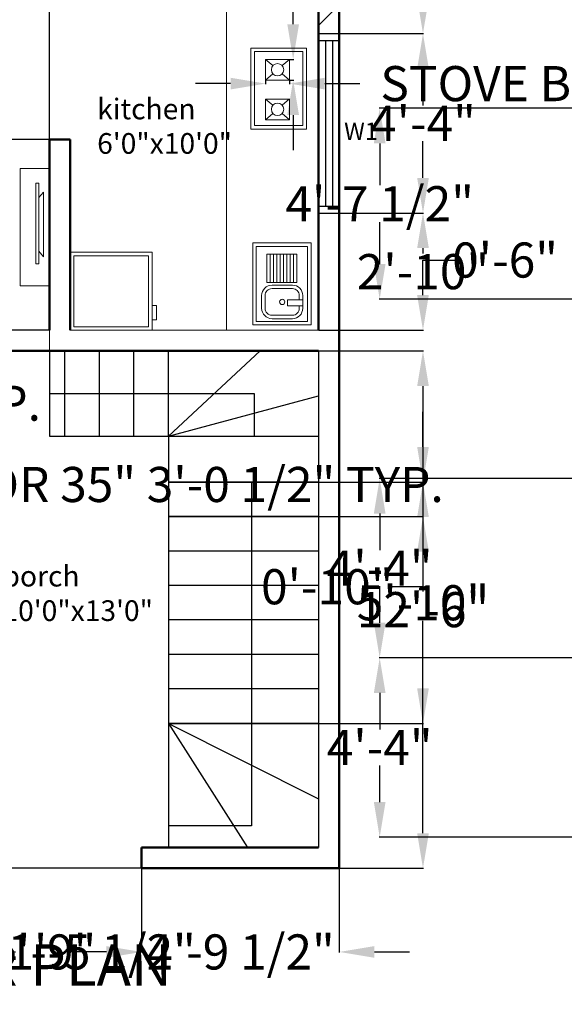
# Model space of a CAD drawing. Units: inches. Extents: x 21 to 3450, y 4 to 2137.
# Tile 10 of 14: x 2964 to 3122, y 1047 to 1333. Entities that reach past the tile are written whole.
import ezdxf

# ---------------------------------------------------------------- set-up
doc = ezdxf.new("R2010")
doc.units = ezdxf.units.IN
doc.header["$MEASUREMENT"] = 0
for name, color, linetype, lineweight in [('A-ANNO-DIMS', 2, 'Continuous', 18), ('A-ANNO-TEXT', 7, 'Continuous', 18), ('A-AREA-IDEN', 3, 'Continuous', 18), ('A-FLOR-FIXT', 9, 'Continuous', 18), ('A-FLOR-STRS', 2, 'Continuous', 25), ('A-FURN', 8, 'Continuous', 18), ('A-GLAZ', 3, 'Continuous', 25), ('A-WALL', 7, 'Continuous', 50), ('A-WALL-PATT', 8, 'Continuous', 13)]:
    doc.layers.add(name, color=color, linetype=linetype, lineweight=lineweight)
doc.styles.get("Standard").update_dxf_attribs({"font": 'arial.ttf'})
doc.dimstyles.get("Standard").update_dxf_attribs({"dimtxt": 10.18, "dimasz": 10.18, "dimexe": 0.18, "dimexo": 0.0625, "dimgap": 0.09, "dimtad": 0, "dimtih": 1, "dimtoh": 1, "dimdec": 0, "dimzin": 0, "dimdsep": 46, "dimlunit": 3, "dimtxsty": 'Standard', "dimcen": 0.09, "dimadec": 0, "dimazin": 0, "dimtfac": 1, "dimtdec": 0, "dimtofl": 0, "dimtmove": 0, "dimatfit": 3, "dimfxl": 1, "dimtolj": 1, "dimtzin": 0, "dimarcsym": 0})

# ---------------------------------------------------------------- blocks, each defined once
blk = doc.blocks.new('*D8')
at = {"layer": 'A-ANNO-DIMS', "color": 0, "lineweight": -2, "transparency": 16777216}
for p, q in [((2816.85, 1506.81), (2803.73, 1506.81)), ((2803.91, 1496.63), (2803.91, 1302.07)), ((2803.91, 1096.92), (2803.91, 1291.48)), ((2999.5, 1086.74), (2803.73, 1086.74))]:
    blk.add_line(p, q, dxfattribs=at)
at = {"layer": 'A-ANNO-DIMS', "color": 0, "transparency": 16777216}
for points in [[(2802.22, 1496.63), (2805.61, 1496.63), (2803.91, 1506.81)], [(2802.22, 1096.92), (2805.61, 1096.92), (2803.91, 1086.74)]]:
    blk.add_solid(points, dxfattribs=at)
at = {"layer": 'Defpoints', "color": 0, "transparency": 16777216}
for p in [(2816.91, 1506.81), (2803.91, 1086.74), (2999.56, 1086.74)]:
    blk.add_point(p, dxfattribs=at)
at = {"layer": 'A-ANNO-DIMS', "color": 0, "transparency": 16777216, "insert": (2803.91, 1296.77), "char_height": 10.18, "attachment_point": 5}
blk.add_mtext("\\A1;35'", dxfattribs=at)
blk = doc.blocks.new('STOVE-BURNER')
blk.add_line((0, 5.99), (2.12, 4.17))
blk.add_lwpolyline([(0, 5.99), (0, 5.99), (6.94, 5.99), (6.94, 5.99), (6.94, 0), (6.94, 0), (0, 0), (0, 0)], close=True)
blk = doc.blocks.new('*D26')
at = {"layer": 'A-ANNO-DIMS', "color": 0, "lineweight": -2, "transparency": 16777216}
for p, q in [((2885.64, 1203.41), (2885.64, 1197.85)), ((2921.91, 1203.41), (2921.91, 1197.85)), ((2895.82, 1198.03), (2911.73, 1198.03)), ((2921.91, 1198.03), (2932.09, 1198.03))]:
    blk.add_line(p, q, dxfattribs=at)
at = {"layer": 'A-ANNO-DIMS', "color": 0, "transparency": 16777216}
for points in [[(2895.82, 1199.72), (2895.82, 1196.33), (2885.64, 1198.03)], [(2911.73, 1199.72), (2911.73, 1196.33), (2921.91, 1198.03)]]:
    blk.add_solid(points, dxfattribs=at)
at = {"layer": 'Defpoints', "color": 0, "transparency": 16777216}
for p in [(2885.64, 1203.47), (2921.91, 1203.47), (2921.91, 1198.03)]:
    blk.add_point(p, dxfattribs=at)
at = {"layer": 'A-ANNO-DIMS', "color": 0, "transparency": 16777216, "insert": (3010.53, 1198.03), "char_height": 10.18, "attachment_point": 5}
blk.add_mtext('\\A1;DOOR 35" 3\'-0 1/2" TYP.', dxfattribs=at)
blk = doc.blocks.new('*D27')
at = {"layer": 'A-ANNO-DIMS', "color": 0, "lineweight": -2, "transparency": 16777216}
for p, q in [((2921.97, 1239.74), (2927.53, 1239.74)), ((2927.35, 1229.56), (2927.35, 1226.96)), ((2927.35, 1213.65), (2927.35, 1216.25)), ((2921.97, 1203.47), (2927.53, 1203.47))]:
    blk.add_line(p, q, dxfattribs=at)
at = {"layer": 'A-ANNO-DIMS', "color": 0, "transparency": 16777216}
for points in [[(2925.66, 1229.56), (2929.05, 1229.56), (2927.35, 1239.74)], [(2925.66, 1213.65), (2929.05, 1213.65), (2927.35, 1203.47)]]:
    blk.add_solid(points, dxfattribs=at)
at = {"layer": 'Defpoints', "color": 0, "transparency": 16777216}
for p in [(2921.91, 1239.74), (2927.35, 1239.74), (2921.91, 1203.47)]:
    blk.add_point(p, dxfattribs=at)
at = {"layer": 'A-ANNO-DIMS', "color": 0, "transparency": 16777216, "insert": (2927.35, 1221.61), "char_height": 10.18, "attachment_point": 5}
blk.add_mtext('\\A1;3\'-0 1/2" TYP.', dxfattribs=at)
blk = doc.blocks.new('*D32')
at = {"layer": 'A-ANNO-DIMS', "color": 0, "lineweight": -2, "transparency": 16777216}
for p, q in [((3025.36, 1314.25), (3015.18, 1314.25)), ((3035.54, 1315.23), (3035.54, 1314.07)), ((3042.48, 1315.23), (3042.48, 1314.07)), ((3052.66, 1314.25), (3062.84, 1314.25))]:
    blk.add_line(p, q, dxfattribs=at)
at = {"layer": 'A-ANNO-DIMS', "color": 0, "transparency": 16777216}
for points in [[(3025.36, 1315.95), (3025.36, 1312.56), (3035.54, 1314.25)], [(3052.66, 1315.95), (3052.66, 1312.56), (3042.48, 1314.25)]]:
    blk.add_solid(points, dxfattribs=at)
at = {"layer": 'Defpoints', "color": 0, "transparency": 16777216}
for p in [(3035.54, 1315.29), (3042.48, 1315.29), (3042.48, 1314.25)]:
    blk.add_point(p, dxfattribs=at)
at = {"layer": 'A-ANNO-DIMS', "color": 0, "transparency": 16777216, "insert": (3152.02, 1314.25), "char_height": 10.18, "attachment_point": 5}
blk.add_mtext('\\A1;STOVE BURNER 0\'-7" TYP.', dxfattribs=at)
blk = doc.blocks.new('*D33')
at = {"layer": 'A-ANNO-DIMS', "color": 0, "lineweight": -2, "transparency": 16777216}
for p, q in [((3043.53, 1331.47), (3043.53, 1341.65)), ((3043.53, 1341.65), (3053.71, 1341.65)), ((3042.55, 1321.29), (3043.71, 1321.29)), ((3042.55, 1315.29), (3043.71, 1315.29)), ((3043.53, 1305.11), (3043.53, 1294.93))]:
    blk.add_line(p, q, dxfattribs=at)
at = {"layer": 'A-ANNO-DIMS', "color": 0, "transparency": 16777216}
for points in [[(3041.83, 1331.47), (3045.22, 1331.47), (3043.53, 1321.29)], [(3041.83, 1305.11), (3045.22, 1305.11), (3043.53, 1315.29)]]:
    blk.add_solid(points, dxfattribs=at)
at = {"layer": 'Defpoints', "color": 0, "transparency": 16777216}
for p in [(3042.48, 1321.29), (3043.53, 1321.29), (3042.48, 1315.29)]:
    blk.add_point(p, dxfattribs=at)
at = {"layer": 'A-ANNO-DIMS', "color": 0, "transparency": 16777216, "insert": (3084.82, 1341.65), "char_height": 10.18, "attachment_point": 5}
blk.add_mtext('\\A1;0\'-6" TYP.', dxfattribs=at)
blk = doc.blocks.new('*D104')
at = {"layer": 'A-ANNO-DIMS', "color": 0, "lineweight": -2, "transparency": 16777216}
for p, q in [((2924.91, 1092.68), (2924.91, 1062.31)), ((2942.64, 1086.68), (2942.64, 1062.31)), ((2914.73, 1062.49), (2904.55, 1062.49)), ((2952.82, 1062.49), (2963, 1062.49))]:
    blk.add_line(p, q, dxfattribs=at)
at = {"layer": 'A-ANNO-DIMS', "color": 0, "transparency": 16777216}
for points in [[(2914.73, 1064.19), (2914.73, 1060.8), (2924.91, 1062.49)], [(2952.82, 1064.19), (2952.82, 1060.8), (2942.64, 1062.49)]]:
    blk.add_solid(points, dxfattribs=at)
at = {"layer": 'Defpoints', "color": 0, "transparency": 16777216}
for p in [(2924.91, 1092.74), (2942.64, 1086.74), (2942.64, 1062.49)]:
    blk.add_point(p, dxfattribs=at)
at = {"layer": 'A-ANNO-DIMS', "color": 0, "transparency": 16777216, "insert": (2988, 1062.49), "char_height": 10.18, "attachment_point": 5}
blk.add_mtext('\\A1;1\'-5 1/2"', dxfattribs=at)
blk = doc.blocks.new('*D105')
at = {"layer": 'A-ANNO-DIMS', "color": 0, "lineweight": -2, "transparency": 16777216}
for p, q in [((2942.64, 1086.68), (2942.64, 1062.31)), ((2999.56, 1086.68), (2999.56, 1062.31)), ((2952.82, 1062.49), (2957.27, 1062.49)), ((2989.38, 1062.49), (2984.92, 1062.49))]:
    blk.add_line(p, q, dxfattribs=at)
at = {"layer": 'A-ANNO-DIMS', "color": 0, "transparency": 16777216}
for points in [[(2952.82, 1064.19), (2952.82, 1060.8), (2942.64, 1062.49)], [(2989.38, 1064.19), (2989.38, 1060.8), (2999.56, 1062.49)]]:
    blk.add_solid(points, dxfattribs=at)
at = {"layer": 'Defpoints', "color": 0, "transparency": 16777216}
for p in [(2942.64, 1086.74), (2999.56, 1086.74), (2999.56, 1062.49)]:
    blk.add_point(p, dxfattribs=at)
at = {"layer": 'A-ANNO-DIMS', "color": 0, "transparency": 16777216, "insert": (2971.1, 1062.49), "char_height": 10.18, "attachment_point": 5}
blk.add_mtext('\\A1;4\'-9"', dxfattribs=at)
blk = doc.blocks.new('*D106')
at = {"layer": 'A-ANNO-DIMS', "color": 0, "lineweight": -2, "transparency": 16777216}
for p, q in [((2999.56, 1086.68), (2999.56, 1062.31)), ((3056.91, 1086.68), (3056.91, 1062.31)), ((2989.38, 1062.49), (2979.2, 1062.49)), ((3067.09, 1062.49), (3077.27, 1062.49))]:
    blk.add_line(p, q, dxfattribs=at)
at = {"layer": 'A-ANNO-DIMS', "color": 0, "transparency": 16777216}
for points in [[(2989.38, 1064.19), (2989.38, 1060.8), (2999.56, 1062.49)], [(3067.09, 1064.19), (3067.09, 1060.8), (3056.91, 1062.49)]]:
    blk.add_solid(points, dxfattribs=at)
at = {"layer": 'Defpoints', "color": 0, "transparency": 16777216}
for p in [(2999.56, 1086.74), (3056.91, 1086.74), (3056.91, 1062.49)]:
    blk.add_point(p, dxfattribs=at)
at = {"layer": 'A-ANNO-DIMS', "color": 0, "transparency": 16777216, "insert": (3028.24, 1062.49), "char_height": 10.18, "attachment_point": 5}
blk.add_mtext('\\A1;4\'-9 1/2"', dxfattribs=at)
blk = doc.blocks.new('*D107')
at = {"layer": 'A-ANNO-DIMS', "color": 0, "lineweight": -2, "transparency": 16777216}
for p, q in [((3050.97, 1236.74), (3081.34, 1236.74)), ((3081.16, 1226.56), (3081.16, 1167.03)), ((3081.16, 1096.92), (3081.16, 1156.46)), ((3056.97, 1086.74), (3081.34, 1086.74))]:
    blk.add_line(p, q, dxfattribs=at)
at = {"layer": 'A-ANNO-DIMS', "color": 0, "transparency": 16777216}
for points in [[(3079.47, 1226.56), (3082.86, 1226.56), (3081.16, 1236.74)], [(3079.47, 1096.92), (3082.86, 1096.92), (3081.16, 1086.74)]]:
    blk.add_solid(points, dxfattribs=at)
at = {"layer": 'Defpoints', "color": 0, "transparency": 16777216}
for p in [(3050.91, 1236.74), (3081.16, 1236.74), (3056.91, 1086.74)]:
    blk.add_point(p, dxfattribs=at)
at = {"layer": 'A-ANNO-DIMS', "color": 0, "transparency": 16777216, "insert": (3081.16, 1161.74), "char_height": 10.18, "attachment_point": 5}
blk.add_mtext('\\A1;12\'-6"', dxfattribs=at)
blk = doc.blocks.new('*D108')
at = {"layer": 'A-ANNO-DIMS', "color": 0, "lineweight": -2, "transparency": 16777216}
for p, q in [((3081.16, 1252.92), (3081.16, 1263.1)), ((3081.16, 1263.1), (3091.34, 1263.1)), ((3050.97, 1242.74), (3081.34, 1242.74)), ((3050.97, 1236.74), (3081.34, 1236.74)), ((3081.16, 1226.56), (3081.16, 1216.38))]:
    blk.add_line(p, q, dxfattribs=at)
at = {"layer": 'A-ANNO-DIMS', "color": 0, "transparency": 16777216}
for points in [[(3079.47, 1252.92), (3082.86, 1252.92), (3081.16, 1242.74)], [(3079.47, 1226.56), (3082.86, 1226.56), (3081.16, 1236.74)]]:
    blk.add_solid(points, dxfattribs=at)
at = {"layer": 'Defpoints', "color": 0, "transparency": 16777216}
for p in [(3050.91, 1242.74), (3081.16, 1242.74), (3050.91, 1236.74)]:
    blk.add_point(p, dxfattribs=at)
at = {"layer": 'A-ANNO-DIMS', "color": 0, "transparency": 16777216, "insert": (3104.96, 1263.1), "char_height": 10.18, "attachment_point": 5}
blk.add_mtext('\\A1;0\'-6"', dxfattribs=at)
blk = doc.blocks.new('*D109')
at = {"layer": 'A-ANNO-DIMS', "color": 0, "lineweight": -2, "transparency": 16777216}
for p, q in [((3056.97, 1276.74), (3081.34, 1276.74)), ((3081.16, 1266.56), (3081.16, 1265.03)), ((3081.16, 1252.92), (3081.16, 1254.46)), ((3050.97, 1242.74), (3081.34, 1242.74))]:
    blk.add_line(p, q, dxfattribs=at)
at = {"layer": 'A-ANNO-DIMS', "color": 0, "transparency": 16777216}
for points in [[(3079.47, 1266.56), (3082.86, 1266.56), (3081.16, 1276.74)], [(3079.47, 1252.92), (3082.86, 1252.92), (3081.16, 1242.74)]]:
    blk.add_solid(points, dxfattribs=at)
at = {"layer": 'Defpoints', "color": 0, "transparency": 16777216}
for p in [(3056.91, 1276.74), (3081.16, 1276.74), (3050.91, 1242.74)]:
    blk.add_point(p, dxfattribs=at)
at = {"layer": 'A-ANNO-DIMS', "color": 0, "transparency": 16777216, "insert": (3081.16, 1259.74), "char_height": 10.18, "attachment_point": 5}
blk.add_mtext('\\A1;2\'-10"', dxfattribs=at)
blk = doc.blocks.new('*D110')
at = {"layer": 'A-ANNO-DIMS', "color": 0, "lineweight": -2, "transparency": 16777216}
for p, q in [((3056.97, 1328.74), (3081.34, 1328.74)), ((3081.16, 1318.56), (3081.16, 1307.92)), ((3081.16, 1286.92), (3081.16, 1297.56)), ((3056.97, 1276.74), (3081.34, 1276.74))]:
    blk.add_line(p, q, dxfattribs=at)
at = {"layer": 'A-ANNO-DIMS', "color": 0, "transparency": 16777216}
for points in [[(3079.47, 1318.56), (3082.86, 1318.56), (3081.16, 1328.74)], [(3079.47, 1286.92), (3082.86, 1286.92), (3081.16, 1276.74)]]:
    blk.add_solid(points, dxfattribs=at)
at = {"layer": 'Defpoints', "color": 0, "transparency": 16777216}
for p in [(3056.91, 1328.74), (3081.16, 1328.74), (3056.91, 1276.74)]:
    blk.add_point(p, dxfattribs=at)
at = {"layer": 'A-ANNO-DIMS', "color": 0, "transparency": 16777216, "insert": (3081.16, 1302.74), "char_height": 10.18, "attachment_point": 5}
blk.add_mtext('\\A1;4\'-4"', dxfattribs=at)
blk = doc.blocks.new('*D111')
at = {"layer": 'A-ANNO-DIMS', "color": 0, "lineweight": -2, "transparency": 16777216}
for p, q in [((3050.97, 1362.74), (3081.34, 1362.74)), ((3081.16, 1352.56), (3081.16, 1351.03)), ((3081.16, 1338.92), (3081.16, 1340.46)), ((3056.97, 1328.74), (3081.34, 1328.74))]:
    blk.add_line(p, q, dxfattribs=at)
at = {"layer": 'A-ANNO-DIMS', "color": 0, "transparency": 16777216}
for points in [[(3079.47, 1352.56), (3082.86, 1352.56), (3081.16, 1362.74)], [(3079.47, 1338.92), (3082.86, 1338.92), (3081.16, 1328.74)]]:
    blk.add_solid(points, dxfattribs=at)
at = {"layer": 'Defpoints', "color": 0, "transparency": 16777216}
for p in [(3050.91, 1362.74), (3081.16, 1362.74), (3056.91, 1328.74)]:
    blk.add_point(p, dxfattribs=at)
at = {"layer": 'A-ANNO-DIMS', "color": 0, "transparency": 16777216, "insert": (3081.16, 1345.74), "char_height": 10.18, "attachment_point": 5}
blk.add_mtext('\\A1;2\'-10"', dxfattribs=at)
blk = doc.blocks.new('*D118')
at = {"layer": 'A-ANNO-DIMS', "color": 0, "lineweight": -2, "transparency": 16777216}
for p, q in [((2920.73, 1539.16), (2910.55, 1539.16)), ((2930.91, 1242.81), (2930.91, 1539.34)), ((2972.91, 1242.81), (2972.91, 1539.34)), ((2983.09, 1539.16), (2993.27, 1539.16))]:
    blk.add_line(p, q, dxfattribs=at)
at = {"layer": 'A-ANNO-DIMS', "color": 0, "transparency": 16777216}
for points in [[(2920.73, 1540.85), (2920.73, 1537.46), (2930.91, 1539.16)], [(2983.09, 1540.85), (2983.09, 1537.46), (2972.91, 1539.16)]]:
    blk.add_solid(points, dxfattribs=at)
at = {"layer": 'Defpoints', "color": 0, "transparency": 16777216}
for p in [(2972.91, 1539.16), (2930.91, 1242.74), (2972.91, 1242.74)]:
    blk.add_point(p, dxfattribs=at)
at = {"layer": 'A-ANNO-DIMS', "color": 0, "transparency": 16777216, "insert": (2951.91, 1539.16), "char_height": 10.18, "attachment_point": 5}
blk.add_mtext('\\A1;3\'-6"', dxfattribs=at)
blk = doc.blocks.new('*D120')
at = {"layer": 'A-ANNO-DIMS', "color": 0, "lineweight": -2, "transparency": 16777216}
for p, q in [((2972.85, 1298.07), (2738.48, 1298.07)), ((2738.66, 1287.89), (2738.66, 1275.76)), ((2738.66, 1252.92), (2738.66, 1265.05)), ((2972.85, 1242.74), (2738.48, 1242.74))]:
    blk.add_line(p, q, dxfattribs=at)
at = {"layer": 'A-ANNO-DIMS', "color": 0, "transparency": 16777216}
for points in [[(2736.97, 1287.89), (2740.36, 1287.89), (2738.66, 1298.07)], [(2736.97, 1252.92), (2740.36, 1252.92), (2738.66, 1242.74)]]:
    blk.add_solid(points, dxfattribs=at)
at = {"layer": 'Defpoints', "color": 0, "transparency": 16777216}
for p in [(2738.66, 1298.07), (2972.91, 1298.07), (2972.91, 1242.74)]:
    blk.add_point(p, dxfattribs=at)
at = {"layer": 'A-ANNO-DIMS', "color": 0, "transparency": 16777216, "insert": (2738.66, 1270.41), "char_height": 10.18, "attachment_point": 5}
blk.add_mtext('\\A1;4\'-7 1/2"', dxfattribs=at)
blk = doc.blocks.new('*D121')
at = {"layer": 'A-ANNO-DIMS', "color": 0, "lineweight": -2, "transparency": 16777216}
for p, q in [((3081.16, 1208.92), (3081.16, 1219.1)), ((3007.42, 1198.74), (3081.34, 1198.74)), ((3007.42, 1188.74), (3081.34, 1188.74)), ((3081.16, 1178.56), (3081.16, 1168.38)), ((3081.16, 1168.38), (3070.98, 1168.38))]:
    blk.add_line(p, q, dxfattribs=at)
at = {"layer": 'A-ANNO-DIMS', "color": 0, "transparency": 16777216}
for points in [[(3079.47, 1208.92), (3082.86, 1208.92), (3081.16, 1198.74)], [(3079.47, 1178.56), (3082.86, 1178.56), (3081.16, 1188.74)]]:
    blk.add_solid(points, dxfattribs=at)
at = {"layer": 'Defpoints', "color": 0, "transparency": 16777216}
for p in [(3007.36, 1198.74), (3007.36, 1188.74), (3081.16, 1188.74)]:
    blk.add_point(p, dxfattribs=at)
at = {"layer": 'A-ANNO-DIMS', "color": 0, "transparency": 16777216, "insert": (3053.41, 1168.38), "char_height": 10.18, "attachment_point": 5}
blk.add_mtext('\\A1;0\'-10"', dxfattribs=at)
blk = doc.blocks.new('*D122')
at = {"layer": 'A-ANNO-DIMS', "color": 0, "lineweight": -2, "transparency": 16777216}
for p, q in [((3007.42, 1198.74), (3081.34, 1198.74)), ((3081.16, 1188.56), (3081.16, 1169.03)), ((3081.16, 1138.92), (3081.16, 1158.46)), ((3007.42, 1128.74), (3081.34, 1128.74))]:
    blk.add_line(p, q, dxfattribs=at)
at = {"layer": 'A-ANNO-DIMS', "color": 0, "transparency": 16777216}
for points in [[(3079.47, 1188.56), (3082.86, 1188.56), (3081.16, 1198.74)], [(3079.47, 1138.92), (3082.86, 1138.92), (3081.16, 1128.74)]]:
    blk.add_solid(points, dxfattribs=at)
at = {"layer": 'Defpoints', "color": 0, "transparency": 16777216}
for p in [(3007.36, 1198.74), (3007.36, 1128.74), (3081.16, 1128.74)]:
    blk.add_point(p, dxfattribs=at)
at = {"layer": 'A-ANNO-DIMS', "color": 0, "transparency": 16777216, "insert": (3081.16, 1163.74), "char_height": 10.18, "attachment_point": 5}
blk.add_mtext('\\A1;5\'-10"', dxfattribs=at)
blk = doc.blocks.new('*D141')
at = {"layer": 'A-ANNO-DIMS', "color": 0, "lineweight": -2, "transparency": 16777216}
for p, q in [((3146.55, 1147.77), (3068.43, 1147.77)), ((3068.61, 1137.59), (3068.61, 1126.95)), ((3068.61, 1105.95), (3068.61, 1116.59)), ((3146.55, 1095.77), (3068.43, 1095.77))]:
    blk.add_line(p, q, dxfattribs=at)
at = {"layer": 'A-ANNO-DIMS', "color": 0, "transparency": 16777216}
for points in [[(3066.91, 1137.59), (3070.31, 1137.59), (3068.61, 1147.77)], [(3066.91, 1105.95), (3070.31, 1105.95), (3068.61, 1095.77)]]:
    blk.add_solid(points, dxfattribs=at)
at = {"layer": 'Defpoints', "color": 0, "transparency": 16777216}
for p in [(3068.61, 1147.77), (3146.61, 1147.77), (3146.61, 1095.77)]:
    blk.add_point(p, dxfattribs=at)
at = {"layer": 'A-ANNO-DIMS', "color": 0, "transparency": 16777216, "insert": (3068.61, 1121.77), "char_height": 10.18, "attachment_point": 5}
blk.add_mtext('\\A1;4\'-4"', dxfattribs=at)
blk = doc.blocks.new('*D142')
at = {"layer": 'A-ANNO-DIMS', "color": 0, "lineweight": -2, "transparency": 16777216}
for p, q in [((3146.55, 1199.77), (3068.43, 1199.77)), ((3068.61, 1189.59), (3068.61, 1178.95)), ((3068.61, 1157.95), (3068.61, 1168.59)), ((3146.55, 1147.77), (3068.43, 1147.77))]:
    blk.add_line(p, q, dxfattribs=at)
at = {"layer": 'A-ANNO-DIMS', "color": 0, "transparency": 16777216}
for points in [[(3066.91, 1189.59), (3070.31, 1189.59), (3068.61, 1199.77)], [(3066.91, 1157.95), (3070.31, 1157.95), (3068.61, 1147.77)]]:
    blk.add_solid(points, dxfattribs=at)
at = {"layer": 'Defpoints', "color": 0, "transparency": 16777216}
for p in [(3068.61, 1199.77), (3146.61, 1199.77), (3146.61, 1147.77)]:
    blk.add_point(p, dxfattribs=at)
at = {"layer": 'A-ANNO-DIMS', "color": 0, "transparency": 16777216, "insert": (3068.61, 1173.77), "char_height": 10.18, "attachment_point": 5}
blk.add_mtext('\\A1;4\'-4"', dxfattribs=at)
blk = doc.blocks.new('*D147')
at = {"layer": 'A-ANNO-DIMS', "color": 0, "lineweight": -2, "transparency": 16777216}
for p, q in [((3302.55, 1307.09), (3068.43, 1307.09)), ((3068.61, 1296.91), (3068.61, 1284.78)), ((3068.61, 1261.95), (3068.61, 1274.08)), ((3302.55, 1251.77), (3068.43, 1251.77))]:
    blk.add_line(p, q, dxfattribs=at)
at = {"layer": 'A-ANNO-DIMS', "color": 0, "transparency": 16777216}
for points in [[(3066.91, 1296.91), (3070.31, 1296.91), (3068.61, 1307.09)], [(3066.91, 1261.95), (3070.31, 1261.95), (3068.61, 1251.77)]]:
    blk.add_solid(points, dxfattribs=at)
at = {"layer": 'Defpoints', "color": 0, "transparency": 16777216}
for p in [(3068.61, 1307.09), (3302.61, 1307.09), (3302.61, 1251.77)]:
    blk.add_point(p, dxfattribs=at)
at = {"layer": 'A-ANNO-DIMS', "color": 0, "transparency": 16777216, "insert": (3068.61, 1279.43), "char_height": 10.18, "attachment_point": 5}
blk.add_mtext('\\A1;4\'-7 1/2"', dxfattribs=at)

msp = doc.modelspace()

# ---------------------------------------------------------------- hatches: boundary and pattern name
at = {"layer": 'A-WALL-PATT'}
h = msp.add_hatch(dxfattribs=at)
h.set_pattern_fill('ANSI31', color=256, scale=46)
h.set_pattern_definition([(45, (-32.016, 151.0237), (-4.065864, 4.065864), [])])
h.paths.add_polyline_path([(2951.41, 1506.74), (2816.91, 1506.74), (2816.91, 1190.74), (2822.91, 1190.74), (2822.91, 1236.74), (2822.91, 1242.74), (2822.91, 1362.74), (2822.91, 1368.74), (2822.91, 1452.74), (2846.41, 1452.74), (2846.41, 1458.74), (2822.91, 1458.74), (2822.91, 1500.74), (2897.91, 1500.74), (2903.91, 1500.74), (2951.41, 1500.74)])
h.paths.add_polyline_path([(3056.91, 1506.74), (3003.41, 1506.74), (3003.41, 1500.74), (3050.91, 1500.74), (3050.91, 1460.31, -0.065004), (3051.05, 1459.28), (3051.05, 1422.47, -0.065004), (3050.91, 1421.45), (3050.91, 1368.74), (2942.4, 1368.74), (2942.4, 1365.74), (2944.4, 1365.74), (2944.4, 1362.74), (2972.91, 1362.74), (2972.91, 1336.29), (2978.91, 1336.29), (2978.91, 1362.74), (3050.91, 1362.74), (3050.91, 1328.74), (3056.91, 1328.74)])
h.paths.add_polyline_path([(2885.91, 1239.74), (2885.91, 1242.74), (2852.91, 1242.74), (2852.91, 1324.17), (2846.91, 1324.17), (2846.91, 1242.74), (2846.91, 1236.74), (2885.91, 1236.74), (2885.91, 1237.74, -0.014283)], flags=17)
h.paths.add_polyline_path([(2847.91, 1092.74), (2822.91, 1092.74), (2822.91, 1138.74), (2816.91, 1138.74), (2816.91, 1086.74), (2847.91, 1086.74)])
h.paths.add_polyline_path([(2911.4, 1368.74), (2903.91, 1368.74), (2897.91, 1368.74), (2846.91, 1368.74), (2846.91, 1362.74), (2852.91, 1362.74), (2903.91, 1362.74), (2911.4, 1362.74)], flags=17)
h.paths.add_polyline_path([(2903.91, 1458.74), (2897.91, 1458.74), (2874.41, 1458.74), (2874.41, 1452.74), (2897.91, 1452.74), (2897.91, 1401.74), (2898.91, 1401.74, -0.017236), (2900.91, 1401.74), (2903.91, 1401.74), (2903.91, 1452.74)], flags=17)

# ---------------------------------------------------------------- linework, layer by layer
at = {"layer": 'A-FLOR-FIXT'}
for p, q in [((3024.16, 1242.74), (3024.16, 1340.31)), ((3042.48, 1321.29), (3040.37, 1319.46)), ((3035.54, 1315.29), (3037.66, 1317.12)), ((3042.48, 1315.29), (3040.37, 1317.12)), ((3042.48, 1309.8), (3040.37, 1307.97)), ((3035.54, 1303.8), (3037.66, 1305.63)), ((3042.48, 1303.8), (3040.37, 1305.63))]:
    msp.add_line(p, q, dxfattribs=at)
for points in [[(3031.27, 1324.56), (3031.27, 1324.56), (3047.36, 1324.56), (3047.36, 1324.56), (3047.36, 1301.09), (3047.36, 1301.09), (3031.27, 1301.09), (3031.27, 1301.09)], [(3032.27, 1323.56), (3046.36, 1323.56), (3046.36, 1302.09), (3032.27, 1302.09)], [(3048.7, 1268.05), (3031.82, 1268.05), (3031.82, 1244.29), (3048.7, 1244.29)], [(2978.91, 1242.74), (2978.91, 1242.74), (3002.6, 1242.74), (3002.6, 1242.74), (3002.6, 1265.35), (3002.6, 1265.35), (2978.91, 1265.35), (2978.91, 1265.35)], [(3047.7, 1267.05), (3047.7, 1267.05), (3032.82, 1267.05), (3032.82, 1267.05), (3032.82, 1245.29), (3032.82, 1245.29), (3047.7, 1245.29), (3047.7, 1245.29)], [(3035.86, 1264.76), (3035.86, 1264.76), (3036.82, 1264.76), (3036.82, 1264.76), (3036.82, 1256.56), (3036.82, 1256.56), (3035.86, 1256.56), (3035.86, 1256.56)], [(3036.82, 1264.76), (3036.82, 1264.76), (3037.79, 1264.76), (3037.79, 1264.76), (3037.79, 1256.56), (3037.79, 1256.56), (3036.82, 1256.56), (3036.82, 1256.56)], [(3037.79, 1264.76), (3037.79, 1264.76), (3038.75, 1264.76), (3038.75, 1264.76), (3038.75, 1256.56), (3038.75, 1256.56), (3037.79, 1256.56), (3037.79, 1256.56)], [(3038.75, 1264.76), (3038.75, 1264.76), (3039.72, 1264.76), (3039.72, 1264.76), (3039.72, 1256.56), (3039.72, 1256.56), (3038.75, 1256.56), (3038.75, 1256.56)], [(3039.72, 1264.76), (3039.72, 1264.76), (3040.69, 1264.76), (3040.69, 1264.76), (3040.69, 1256.56), (3040.69, 1256.56), (3039.72, 1256.56), (3039.72, 1256.56)], [(3040.69, 1264.76), (3040.69, 1264.76), (3041.65, 1264.76), (3041.65, 1264.76), (3041.65, 1256.56), (3041.65, 1256.56), (3040.69, 1256.56), (3040.69, 1256.56)], [(3041.65, 1264.76), (3041.65, 1264.76), (3042.62, 1264.76), (3042.62, 1264.76), (3042.62, 1256.56), (3042.62, 1256.56), (3041.65, 1256.56), (3041.65, 1256.56)], [(3042.62, 1264.76), (3042.62, 1264.76), (3043.58, 1264.76), (3043.58, 1264.76), (3043.58, 1256.56), (3043.58, 1256.56), (3042.62, 1256.56), (3042.62, 1256.56)], [(3043.58, 1264.76), (3043.58, 1264.76), (3044.55, 1264.76), (3044.55, 1264.76), (3044.55, 1256.56), (3044.55, 1256.56), (3043.58, 1256.56), (3043.58, 1256.56)], [(2979.91, 1243.74), (3001.6, 1243.74), (3001.6, 1264.35), (2979.91, 1264.35)], [(3046.31, 1251.61), (3046.31, 1251.61), (3041.91, 1251.61), (3041.91, 1251.61), (3041.91, 1249.8), (3041.91, 1249.8), (3046.31, 1249.8), (3046.31, 1249.8)], [(3002.6, 1245.72), (3002.6, 1245.72), (3003.92, 1245.72), (3003.92, 1245.72), (3003.92, 1249.88), (3003.92, 1249.88), (3002.6, 1249.88), (3002.6, 1249.88)]]:
    msp.add_lwpolyline(points, close=True, dxfattribs=at)
msp.add_lwpolyline([(3034.39, 1252.81, -0.414214), (3037.39, 1255.81), (3043.31, 1255.81, -0.414214), (3046.31, 1252.81), (3046.31, 1249.1, -0.414214), (3043.31, 1246.1), (3037.39, 1246.1, -0.414214), (3034.39, 1249.1)], format="xyb", close=True, dxfattribs=at)
msp.add_lwpolyline([(3045.31, 1249.8), (3045.31, 1249.1, -0.414214), (3043.31, 1247.1), (3037.39, 1247.1, -0.414214), (3035.39, 1249.1), (3035.39, 1252.81, -0.414214), (3037.39, 1254.81), (3043.31, 1254.81, -0.414214), (3045.31, 1252.81), (3045.31, 1251.61)], format="xyb", dxfattribs=at)
for centre, radius in [((3039.01, 1318.29), 1.79), ((3039.01, 1306.8), 1.79), ((3040.35, 1250.95), 0.767)]:
    msp.add_circle(centre, radius, dxfattribs=at)
at = {"layer": 'A-FLOR-STRS'}
for p, q in [((2972.91, 1236.74), (2972.91, 1212.04)), ((2977.36, 1212.04), (2977.36, 1236.74)), ((2987.36, 1212.04), (2987.36, 1236.74)), ((2997.36, 1212.04), (2997.36, 1236.74)), ((3007.36, 1212.04), (3007.36, 1236.74)), ((3007.36, 1212.04), (3033.97, 1236.74)), ((3050.91, 1236.74), (3050.91, 1092.74)), ((2972.91, 1224.39), (3032.21, 1224.39)), ((3007.36, 1212.04), (3050.91, 1223.71)), ((3032.21, 1224.39), (3032.21, 1212.04)), ((2972.91, 1212.04), (3007.36, 1212.04)), ((3007.36, 1212.04), (3007.36, 1092.74)), ((3007.36, 1212.04), (3050.91, 1212.04)), ((3050.91, 1198.74), (3007.36, 1198.74)), ((3031.47, 1198.74), (3031.47, 1099.07)), ((3050.91, 1188.74), (3007.36, 1188.74)), ((3050.91, 1188.74), (3007.36, 1188.74)), ((3050.91, 1178.74), (3007.36, 1178.74)), ((3050.91, 1168.74), (3007.36, 1168.74)), ((3050.91, 1158.74), (3007.36, 1158.74)), ((3050.91, 1148.74), (3007.36, 1148.74)), ((3050.91, 1138.74), (3007.36, 1138.74)), ((3050.91, 1128.74), (3007.36, 1128.74)), ((3007.36, 1128.74), (3050.91, 1106.87)), ((3007.36, 1128.74), (3030.32, 1092.74)), ((3031.47, 1099.07), (3007.36, 1099.07))]:
    msp.add_line(p, q, dxfattribs=at)
at = {"layer": 'A-FURN'}
for p, q in [((2969.81, 1281.21), (2971.18, 1282.75)), ((2971.18, 1282.75), (2971.18, 1264.07)), ((2971.18, 1264.07), (2969.81, 1265.7)), ((2972.91, 1242.74), (2972.91, 1236.74)), ((2978.91, 1242.74), (3050.91, 1242.74))]:
    msp.add_line(p, q, dxfattribs=at)
for points in [[(2972.91, 1289.66), (2972.91, 1289.66), (2964.34, 1289.66), (2964.34, 1289.66), (2964.34, 1255.66), (2964.34, 1255.66), (2972.91, 1255.66), (2972.91, 1255.66)], [(2969.81, 1285.41), (2969.81, 1285.41), (2968.87, 1285.41), (2968.87, 1285.41), (2968.87, 1262.02), (2968.87, 1262.02), (2969.81, 1262.02), (2969.81, 1262.02)]]:
    msp.add_lwpolyline(points, close=True, dxfattribs=at)
at = {"layer": 'A-GLAZ'}
for p, q in [((3050.91, 1328.74), (3056.91, 1328.74)), ((3050.91, 1326.74), (3056.91, 1326.74)), ((3052.91, 1326.74), (3052.91, 1278.74)), ((3054.91, 1326.74), (3054.91, 1278.74)), ((3050.91, 1278.74), (3056.91, 1278.74)), ((3050.91, 1276.74), (3056.91, 1276.74))]:
    msp.add_line(p, q, dxfattribs=at)
at = {"layer": 'A-WALL'}
for p, q in [((3056.91, 1506.74), (3056.91, 1086.74)), ((3050.91, 1362.74), (3050.91, 1242.74)), ((2972.91, 1298.07), (2978.91, 1298.07)), ((2972.91, 1298.07), (2972.91, 1242.74)), ((2978.91, 1298.07), (2978.91, 1242.74)), ((2930.91, 1236.74), (3050.91, 1236.74)), ((3050.91, 1092.74), (2999.56, 1092.74)), ((2999.56, 1092.74), (2999.56, 1086.74)), ((3056.91, 1086.74), (2999.56, 1086.74))]:
    msp.add_line(p, q, dxfattribs=at)

# ---------------------------------------------------------------- block references
at = {"layer": 'A-FLOR-FIXT'}
for p in [(3035.54, 1315.29), (3035.54, 1303.8)]:
    msp.add_blockref('STOVE-BURNER', p, dxfattribs=at)

# ---------------------------------------------------------------- texts
at = {"layer": 'A-ANNO-TEXT', "attachment_point": 1}
for s, width, insert, char_height in [('W1', 14.628, (3058.3, 1302.94), 5), ('GROUND FLOOR PLAN', 189.6067, (2838.61, 1064.72), 12)]:
    msp.add_mtext_dynamic_manual_height_columns(s, width=width, gutter_width=1, heights=[0], dxfattribs=dict(at, insert=insert, char_height=char_height))
at = {"layer": 'A-AREA-IDEN', "char_height": 6, "attachment_point": 1}
for s, insert in [('kitchen\\P6\'0"x10\'0"', (2986.7, 1309.91)), ('porch\\P10\'0"x13\'0"', (2959.24, 1174.45))]:
    msp.add_mtext_dynamic_manual_height_columns(s, width=84.0083, gutter_width=1, heights=[0], dxfattribs=dict(at, insert=insert))

# ---------------------------------------------------------------- dimensions: what is measured, and where the dimension line sits
at = {"layer": 'A-ANNO-DIMS'}
for base, p1, p2, picture, middle in [((2972.91, 1539.16), (2930.91, 1242.74), (2972.91, 1242.74), '*D118', (2951.91, 1539.16)), ((2942.64, 1062.49), (2924.91, 1092.74), (2942.64, 1086.74), '*D104', (2988, 1062.49)), ((2999.56, 1062.49), (2942.64, 1086.74), (2999.56, 1086.74), '*D105', (2971.1, 1062.49)), ((3056.9118, 1062.4936), (2999.5582, 1086.7436), (3056.9118, 1086.7436), '*D106', (3028.235, 1062.4936))]:
    dim = msp.add_linear_dim(base=base, p1=p1, p2=p2, dimstyle='Standard', override={"dimdec": 1, "dimlfac": 1, "dimrnd": 0, "dimzin": 1, "dimdsep": 46, "dimlunit": 4, "dimfrac": 2}, dxfattribs=at)
    dim.commit()
    dim.dimension.update_dxf_attribs({"geometry": picture, "text_midpoint": middle})
for base, p1, p2, override, picture, middle in [((2803.91, 1086.74), (2816.91, 1506.81), (2999.56, 1086.74), {"dimclrd": 0, "dimclre": 0, "dimclrt": 0}, '*D8', (2803.91, 1296.77)), ((3081.16, 1362.74), (3056.91, 1328.74), (3050.91, 1362.74), {"dimdec": 1, "dimlfac": 1, "dimrnd": 0, "dimzin": 1, "dimdsep": 46, "dimlunit": 4, "dimfrac": 2}, '*D111', (3081.16, 1345.74)), ((3081.16, 1328.74), (3056.91, 1276.74), (3056.91, 1328.74), {"dimdec": 1, "dimlfac": 1, "dimrnd": 0, "dimzin": 1, "dimdsep": 46, "dimlunit": 4, "dimfrac": 2}, '*D110', (3081.16, 1302.74)), ((3068.61, 1307.09), (3302.61, 1251.77), (3302.61, 1307.09), {"dimdec": 1, "dimlfac": 1, "dimrnd": 0, "dimzin": 1, "dimdsep": 46, "dimlunit": 4, "dimfrac": 2}, '*D147', (3068.61, 1279.43)), ((2738.66, 1298.07), (2972.91, 1242.74), (2972.91, 1298.07), {"dimdec": 1, "dimlfac": 1, "dimrnd": 0, "dimzin": 1, "dimdsep": 46, "dimlunit": 4, "dimfrac": 2}, '*D120', (2738.66, 1270.41)), ((3081.16, 1276.74), (3050.91, 1242.74), (3056.91, 1276.74), {"dimdec": 1, "dimlfac": 1, "dimrnd": 0, "dimzin": 1, "dimdsep": 46, "dimlunit": 4, "dimfrac": 2}, '*D109', (3081.16, 1259.74)), ((3081.16, 1242.74), (3050.91, 1236.74), (3050.91, 1242.74), {"dimdec": 1, "dimlfac": 1, "dimrnd": 0, "dimzin": 1, "dimdsep": 46, "dimlunit": 4, "dimfrac": 2}, '*D108', (3104.96, 1263.1)), ((3081.16, 1236.74), (3056.91, 1086.74), (3050.91, 1236.74), {"dimdec": 1, "dimlfac": 1, "dimrnd": 0, "dimzin": 1, "dimdsep": 46, "dimlunit": 4, "dimfrac": 2}, '*D107', (3081.16, 1161.74)), ((3081.16, 1188.74), (3007.36, 1198.74), (3007.36, 1188.74), {"dimdec": 1, "dimlfac": 1, "dimrnd": 0, "dimzin": 1, "dimdsep": 46, "dimlunit": 4, "dimfrac": 2}, '*D121', (3053.41, 1168.38)), ((3068.61, 1199.77), (3146.61, 1147.77), (3146.61, 1199.77), {"dimdec": 1, "dimlfac": 1, "dimrnd": 0, "dimzin": 1, "dimdsep": 46, "dimlunit": 4, "dimfrac": 2}, '*D142', (3068.61, 1173.77)), ((3081.16, 1128.74), (3007.36, 1198.74), (3007.36, 1128.74), {"dimdec": 1, "dimlfac": 1, "dimrnd": 0, "dimzin": 1, "dimdsep": 46, "dimlunit": 4, "dimfrac": 2}, '*D122', (3081.16, 1163.74)), ((3068.61, 1147.77), (3146.61, 1095.77), (3146.61, 1147.77), {"dimdec": 1, "dimlfac": 1, "dimrnd": 0, "dimzin": 1, "dimdsep": 46, "dimlunit": 4, "dimfrac": 2}, '*D141', (3068.61, 1121.77))]:
    dim = msp.add_linear_dim(base=base, p1=p1, p2=p2, angle=90, dimstyle='Standard', override=override, dxfattribs=at)
    dim.commit()
    dim.dimension.update_dxf_attribs({"geometry": picture, "text_midpoint": middle})
for base, p1, p2, picture, middle in [((3043.53, 1321.29), (3042.48, 1315.29), (3042.48, 1321.29), '*D33', (3084.82, 1341.65)), ((2927.35, 1239.74), (2921.91, 1203.47), (2921.91, 1239.74), '*D27', (2927.35, 1221.61))]:
    dim = msp.add_linear_dim(base=base, p1=p1, p2=p2, angle=90, text='<> TYP.', dimstyle='Standard', override={"dimdec": 1, "dimrnd": 0, "dimzin": 1, "dimlunit": 4, "dimfrac": 2}, dxfattribs=at)
    dim.commit()
    dim.dimension.update_dxf_attribs({"geometry": picture, "text_midpoint": middle})
for base, p1, p2, text, picture, middle in [((3042.48, 1314.25), (3035.54, 1315.29), (3042.48, 1315.29), 'STOVE BURNER <> TYP.', '*D32', (3152.02, 1314.25)), ((2921.91, 1198.03), (2885.64, 1203.47), (2921.91, 1203.47), 'DOOR 35" <> TYP.', '*D26', (3010.53, 1198.03))]:
    dim = msp.add_linear_dim(base=base, p1=p1, p2=p2, text=text, dimstyle='Standard', override={"dimdec": 1, "dimrnd": 0, "dimzin": 1, "dimlunit": 4, "dimfrac": 2}, dxfattribs=at)
    dim.commit()
    dim.dimension.update_dxf_attribs({"geometry": picture, "text_midpoint": middle})

doc.saveas('drawing.dxf')
